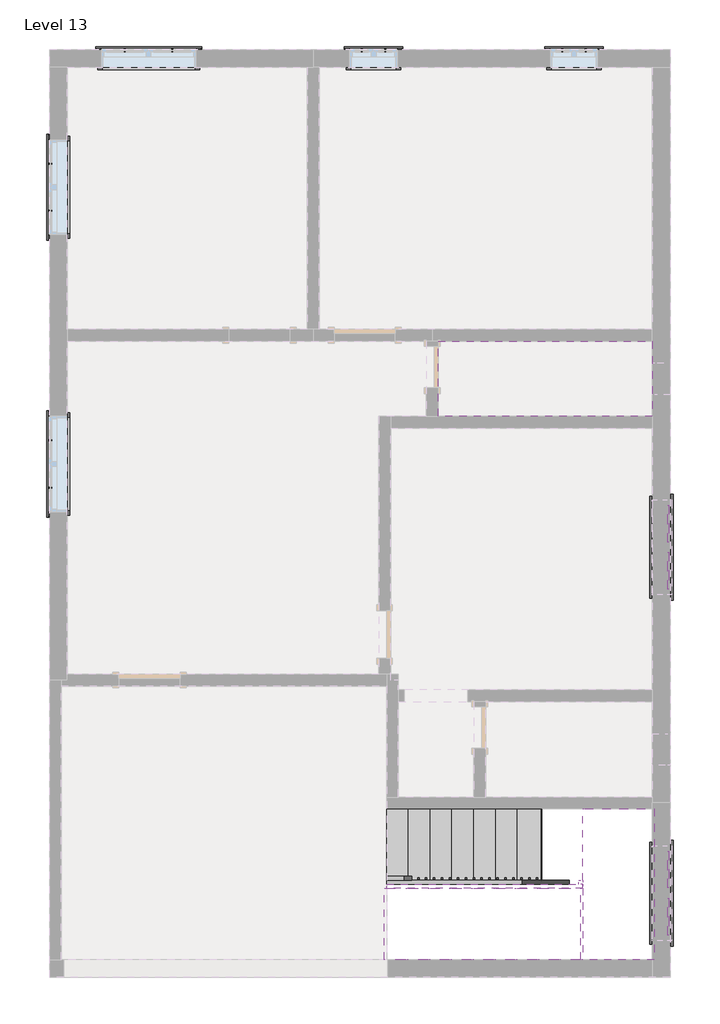
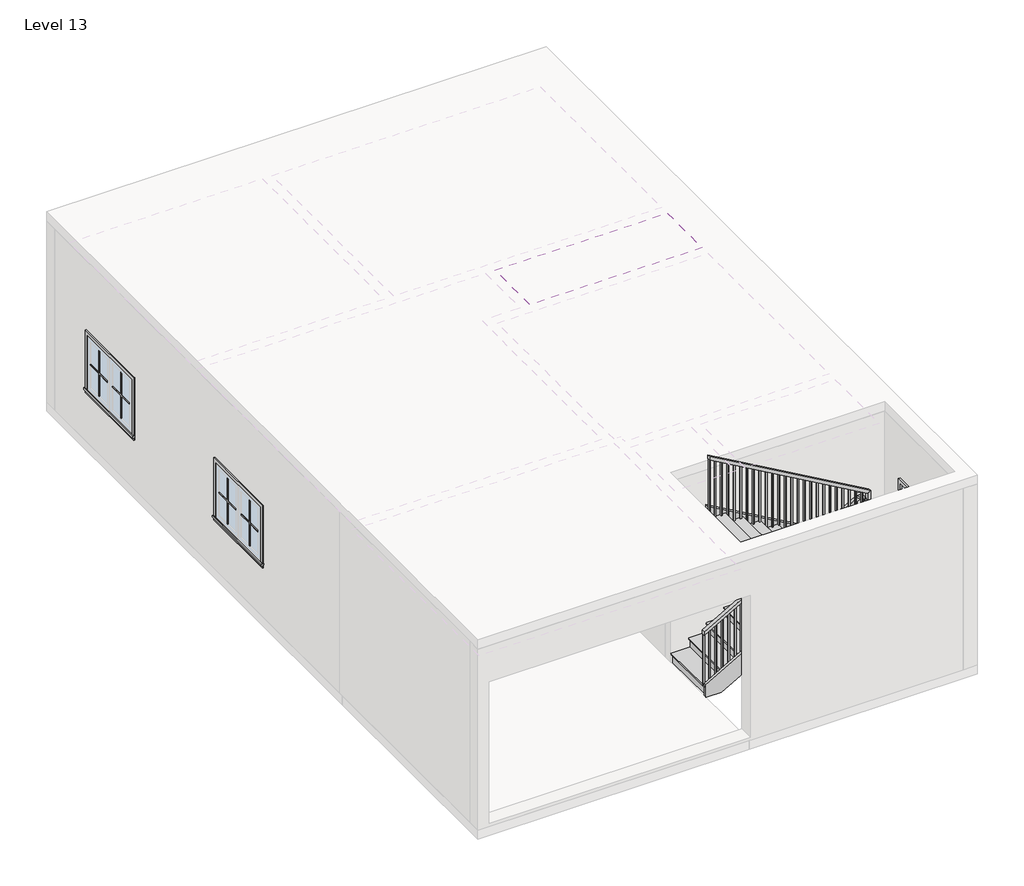
# One storey, part 2 of 2: 44 proxies, 3 members, 2 stair flights, 1 covering, 1 railing, 1 slab.
"""IFC4 building model written with IfcOpenShell, lengths in millimetres."""

from ifc_helpers import new_model, si_unit, frame, origin, place, context, project, spatial, polyline, outline, extrude, faceted_brep, transform, mapped, element, save
from components import muntin_pattern_2x2_muntin_pattern_2x2_2357e71d, muntin_pattern_2x2_muntin_pattern_2x2_302d8f29, muntin_pattern_2x2_muntin_pattern_2x2_53152e2c, muntin_pattern_2x2_muntin_pattern_2x2_e8f3e573, trim_window_exterior_flat_with_sill_c4e67c73, trim_window_exterior_flat_with_sill_a665a915, trim_window_interior_flat_picture_frame_cf1733af, trim_window_interior_flat_picture_frame_d485c387, non_monolithic_landing_4fb2f634, stair_flight_54a58d27, stair_flight_043378c7

model = new_model("IFC4")

# Units and contexts
model_context = context("Model", 3, world=origin())
ifc_project = project(units=[si_unit("LENGTHUNIT", "METRE", prefix="MILLI")], contexts=[model_context])

# Site, building, storey
site = spatial("IfcSite", under=ifc_project)
building = spatial("IfcBuilding", under=site)
storey = spatial("IfcBuildingStorey", under=building, Name="Level 13", Elevation=3200.4)

# Proxies
placement = place(None, origin())
muntin_pattern_2x2_muntin_pattern_2x2_shape = muntin_pattern_2x2_muntin_pattern_2x2_2357e71d(model_context)
element("IfcBuildingElementProxy", 1, Name="Muntin Pattern_2x2 : Muntin Pattern_2x2", ObjectType="Muntin Pattern_2x2 : Muntin Pattern_2x2", at=placement, inside=storey, context=model_context, shape_type="MappedRepresentation", body=[
    mapped(muntin_pattern_2x2_muntin_pattern_2x2_shape, transform((-4942.3279463, 5897.3080275, 4184.65), x_axis=(1.0, 0.0, 0.0), y_axis=(0.0, 1.0, 0.0), z_axis=(0.0, 0.0, 1.0))),
])
element("IfcBuildingElementProxy", 2, Name="Muntin Pattern_2x2 : Muntin Pattern_2x2", ObjectType="Muntin Pattern_2x2 : Muntin Pattern_2x2", at=placement, inside=storey, context=model_context, shape_type="MappedRepresentation", body=[
    mapped(muntin_pattern_2x2_muntin_pattern_2x2_shape, transform((-5899.5904463, 3838.3205275, 4184.65), x_axis=(0.0, 1.0, 0.0), y_axis=(-1.0, 0.0, 0.0), z_axis=(0.0, 0.0, 1.0))),
])
element("IfcBuildingElementProxy", 3, Name="Muntin Pattern_2x2 : Muntin Pattern_2x2", ObjectType="Muntin Pattern_2x2 : Muntin Pattern_2x2", at=placement, inside=storey, context=model_context, shape_type="MappedRepresentation", body=[
    mapped(muntin_pattern_2x2_muntin_pattern_2x2_shape, transform((-5899.5904463, 293.4330275, 4184.65), x_axis=(0.0, 1.0, 0.0), y_axis=(-1.0, 0.0, 0.0), z_axis=(0.0, 0.0, 1.0))),
])
element("IfcBuildingElementProxy", 4, Name="Muntin Pattern_2x2 : Muntin Pattern_2x2", ObjectType="Muntin Pattern_2x2 : Muntin Pattern_2x2", at=placement, inside=storey, context=model_context, shape_type="MappedRepresentation", body=[
    mapped(muntin_pattern_2x2_muntin_pattern_2x2_shape, transform((2031.5595537, -166.9419725, 4489.45), x_axis=(0.0, -1.0, 0.0), y_axis=(1.0, 0.0, 0.0), z_axis=(0.0, 0.0, 1.0))),
])
element("IfcBuildingElementProxy", 5, Name="Muntin Pattern_2x2 : Muntin Pattern_2x2", ObjectType="Muntin Pattern_2x2 : Muntin Pattern_2x2", at=placement, inside=storey, context=model_context, shape_type="MappedRepresentation", body=[
    mapped(muntin_pattern_2x2_muntin_pattern_2x2_shape, transform((2031.5595537, -4599.2419725, 4489.45), x_axis=(0.0, -1.0, 0.0), y_axis=(1.0, 0.0, 0.0), z_axis=(0.0, 0.0, 1.0))),
])
element("IfcBuildingElementProxy", 6, Name="Muntin Pattern_2x2 : Muntin Pattern_2x2", ObjectType="Muntin Pattern_2x2 : Muntin Pattern_2x2", at=placement, inside=storey, context=model_context, shape_type="MappedRepresentation", body=[
    mapped(muntin_pattern_2x2_muntin_pattern_2x2_shape, transform((-4942.3279463, 5897.3080275, 4184.65), x_axis=(1.0, 0.0, 0.0), y_axis=(0.0, 1.0, 0.0), z_axis=(0.0, 0.0, 1.0))),
])
element("IfcBuildingElementProxy", 7, Name="Muntin Pattern_2x2 : Muntin Pattern_2x2", ObjectType="Muntin Pattern_2x2 : Muntin Pattern_2x2", at=placement, inside=storey, context=model_context, shape_type="MappedRepresentation", body=[
    mapped(muntin_pattern_2x2_muntin_pattern_2x2_shape, transform((2031.5595537, -4599.2419725, 4489.45), x_axis=(0.0, -1.0, 0.0), y_axis=(1.0, 0.0, 0.0), z_axis=(0.0, 0.0, 1.0))),
])
muntin_pattern_2x2_muntin_pattern_2x2_2_shape = muntin_pattern_2x2_muntin_pattern_2x2_302d8f29(model_context)
element("IfcBuildingElementProxy", 8, Name="Muntin Pattern_2x2 : Muntin Pattern_2x2", ObjectType="Muntin Pattern_2x2 : Muntin Pattern_2x2", at=placement, inside=storey, context=model_context, shape_type="MappedRepresentation", body=[
    mapped(muntin_pattern_2x2_muntin_pattern_2x2_2_shape, transform((-4335.9029463, 5897.3080275, 4184.65), x_axis=(-1.0, 0.0, 0.0), y_axis=(0.0, -1.0, 0.0), z_axis=(0.0, 0.0, 1.0))),
])
element("IfcBuildingElementProxy", 9, Name="Muntin Pattern_2x2 : Muntin Pattern_2x2", ObjectType="Muntin Pattern_2x2 : Muntin Pattern_2x2", at=placement, inside=storey, context=model_context, shape_type="MappedRepresentation", body=[
    mapped(muntin_pattern_2x2_muntin_pattern_2x2_2_shape, transform((-5899.5904463, 4444.7455275, 4184.65), x_axis=(0.0, -1.0, 0.0), y_axis=(1.0, 0.0, 0.0), z_axis=(0.0, 0.0, 1.0))),
])
element("IfcBuildingElementProxy", 10, Name="Muntin Pattern_2x2 : Muntin Pattern_2x2", ObjectType="Muntin Pattern_2x2 : Muntin Pattern_2x2", at=placement, inside=storey, context=model_context, shape_type="MappedRepresentation", body=[
    mapped(muntin_pattern_2x2_muntin_pattern_2x2_2_shape, transform((-5899.5904463, 899.8580275, 4184.65), x_axis=(0.0, -1.0, 0.0), y_axis=(1.0, 0.0, 0.0), z_axis=(0.0, 0.0, 1.0))),
])
element("IfcBuildingElementProxy", 11, Name="Muntin Pattern_2x2 : Muntin Pattern_2x2", ObjectType="Muntin Pattern_2x2 : Muntin Pattern_2x2", at=placement, inside=storey, context=model_context, shape_type="MappedRepresentation", body=[
    mapped(muntin_pattern_2x2_muntin_pattern_2x2_2_shape, transform((2031.5595537, -773.3669725, 4489.45), x_axis=(0.0, 1.0, 0.0), y_axis=(-1.0, 0.0, 0.0), z_axis=(0.0, 0.0, 1.0))),
])
element("IfcBuildingElementProxy", 12, Name="Muntin Pattern_2x2 : Muntin Pattern_2x2", ObjectType="Muntin Pattern_2x2 : Muntin Pattern_2x2", at=placement, inside=storey, context=model_context, shape_type="MappedRepresentation", body=[
    mapped(muntin_pattern_2x2_muntin_pattern_2x2_2_shape, transform((2031.5595537, -5205.6669725, 4489.45), x_axis=(0.0, 1.0, 0.0), y_axis=(-1.0, 0.0, 0.0), z_axis=(0.0, 0.0, 1.0))),
])
element("IfcBuildingElementProxy", 13, Name="Muntin Pattern_2x2 : Muntin Pattern_2x2", ObjectType="Muntin Pattern_2x2 : Muntin Pattern_2x2", at=placement, inside=storey, context=model_context, shape_type="MappedRepresentation", body=[
    mapped(muntin_pattern_2x2_muntin_pattern_2x2_2_shape, transform((-4335.9029463, 5897.3080275, 4184.65), x_axis=(-1.0, 0.0, 0.0), y_axis=(0.0, -1.0, 0.0), z_axis=(0.0, 0.0, 1.0))),
])
element("IfcBuildingElementProxy", 14, Name="Muntin Pattern_2x2 : Muntin Pattern_2x2", ObjectType="Muntin Pattern_2x2 : Muntin Pattern_2x2", at=placement, inside=storey, context=model_context, shape_type="MappedRepresentation", body=[
    mapped(muntin_pattern_2x2_muntin_pattern_2x2_2_shape, transform((2031.5595537, -5205.6669725, 4489.45), x_axis=(0.0, 1.0, 0.0), y_axis=(-1.0, 0.0, 0.0), z_axis=(0.0, 0.0, 1.0))),
])
muntin_pattern_2x2_muntin_pattern_2x2_3_shape = muntin_pattern_2x2_muntin_pattern_2x2_53152e2c(model_context)
element("IfcBuildingElementProxy", 15, Name="Muntin Pattern_2x2 : Muntin Pattern_2x2", ObjectType="Muntin Pattern_2x2 : Muntin Pattern_2x2", at=placement, inside=storey, context=model_context, shape_type="MappedRepresentation", body=[
    mapped(muntin_pattern_2x2_muntin_pattern_2x2_3_shape, transform((-1907.0279463, 5897.3080275, 4184.65), x_axis=(1.0, 0.0, 0.0), y_axis=(0.0, 1.0, 0.0), z_axis=(0.0, 0.0, 1.0))),
])
element("IfcBuildingElementProxy", 16, Name="Muntin Pattern_2x2 : Muntin Pattern_2x2", ObjectType="Muntin Pattern_2x2 : Muntin Pattern_2x2", at=placement, inside=storey, context=model_context, shape_type="MappedRepresentation", body=[
    mapped(muntin_pattern_2x2_muntin_pattern_2x2_3_shape, transform((658.3720537, 5897.3080275, 4184.65), x_axis=(1.0, 0.0, 0.0), y_axis=(0.0, 1.0, 0.0), z_axis=(0.0, 0.0, 1.0))),
])
element("IfcBuildingElementProxy", 17, Name="Muntin Pattern_2x2 : Muntin Pattern_2x2", ObjectType="Muntin Pattern_2x2 : Muntin Pattern_2x2", at=placement, inside=storey, context=model_context, shape_type="MappedRepresentation", body=[
    mapped(muntin_pattern_2x2_muntin_pattern_2x2_3_shape, transform((-1907.0279463, 5897.3080275, 4184.65), x_axis=(1.0, 0.0, 0.0), y_axis=(0.0, 1.0, 0.0), z_axis=(0.0, 0.0, 1.0))),
])
element("IfcBuildingElementProxy", 18, Name="Muntin Pattern_2x2 : Muntin Pattern_2x2", ObjectType="Muntin Pattern_2x2 : Muntin Pattern_2x2", at=placement, inside=storey, context=model_context, shape_type="MappedRepresentation", body=[
    mapped(muntin_pattern_2x2_muntin_pattern_2x2_3_shape, transform((658.3720537, 5897.3080275, 4184.65), x_axis=(1.0, 0.0, 0.0), y_axis=(0.0, 1.0, 0.0), z_axis=(0.0, 0.0, 1.0))),
])
muntin_pattern_2x2_muntin_pattern_2x2_4_shape = muntin_pattern_2x2_muntin_pattern_2x2_e8f3e573(model_context)
element("IfcBuildingElementProxy", 19, Name="Muntin Pattern_2x2 : Muntin Pattern_2x2", ObjectType="Muntin Pattern_2x2 : Muntin Pattern_2x2", at=placement, inside=storey, context=model_context, shape_type="MappedRepresentation", body=[
    mapped(muntin_pattern_2x2_muntin_pattern_2x2_4_shape, transform((-1605.4029463, 5897.3080275, 4184.65), x_axis=(-1.0, 0.0, 0.0), y_axis=(0.0, -1.0, 0.0), z_axis=(0.0, 0.0, 1.0))),
])
element("IfcBuildingElementProxy", 20, Name="Muntin Pattern_2x2 : Muntin Pattern_2x2", ObjectType="Muntin Pattern_2x2 : Muntin Pattern_2x2", at=placement, inside=storey, context=model_context, shape_type="MappedRepresentation", body=[
    mapped(muntin_pattern_2x2_muntin_pattern_2x2_4_shape, transform((959.9970537, 5897.3080275, 4184.65), x_axis=(-1.0, 0.0, 0.0), y_axis=(0.0, -1.0, 0.0), z_axis=(0.0, 0.0, 1.0))),
])
element("IfcBuildingElementProxy", 21, Name="Muntin Pattern_2x2 : Muntin Pattern_2x2", ObjectType="Muntin Pattern_2x2 : Muntin Pattern_2x2", at=placement, inside=storey, context=model_context, shape_type="MappedRepresentation", body=[
    mapped(muntin_pattern_2x2_muntin_pattern_2x2_4_shape, transform((-1605.4029463, 5897.3080275, 4184.65), x_axis=(-1.0, 0.0, 0.0), y_axis=(0.0, -1.0, 0.0), z_axis=(0.0, 0.0, 1.0))),
])
element("IfcBuildingElementProxy", 22, Name="Muntin Pattern_2x2 : Muntin Pattern_2x2", ObjectType="Muntin Pattern_2x2 : Muntin Pattern_2x2", at=placement, inside=storey, context=model_context, shape_type="MappedRepresentation", body=[
    mapped(muntin_pattern_2x2_muntin_pattern_2x2_4_shape, transform((959.9970537, 5897.3080275, 4184.65), x_axis=(-1.0, 0.0, 0.0), y_axis=(0.0, -1.0, 0.0), z_axis=(0.0, 0.0, 1.0))),
])
trim_window_exterior_flat_with_sill_shape = trim_window_exterior_flat_with_sill_c4e67c73(model_context)
element("IfcBuildingElementProxy", 23, Name="Trim-Window-Exterior-Flat : with Sill", ObjectType="Trim-Window-Exterior-Flat : with Sill", at=placement, inside=storey, context=model_context, shape_type="MappedRepresentation", body=[
    mapped(trim_window_exterior_flat_with_sill_shape, transform((-4639.1154463, 5906.8330275, 5029.2), x_axis=(-1.0, 0.0, 0.0), y_axis=(0.0, 0.0, 1.0), z_axis=(0.0, 1.0, 0.0))),
])
element("IfcBuildingElementProxy", 24, Name="Trim-Window-Exterior-Flat : with Sill", ObjectType="Trim-Window-Exterior-Flat : with Sill", at=placement, inside=storey, context=model_context, shape_type="MappedRepresentation", body=[
    mapped(trim_window_exterior_flat_with_sill_shape, transform((-5909.1154463, 4141.5330275, 5029.2), x_axis=(0.0, -1.0, 0.0), y_axis=(0.0, 0.0, 1.0), z_axis=(-1.0, 0.0, 0.0))),
])
element("IfcBuildingElementProxy", 25, Name="Trim-Window-Exterior-Flat : with Sill", ObjectType="Trim-Window-Exterior-Flat : with Sill", at=placement, inside=storey, context=model_context, shape_type="MappedRepresentation", body=[
    mapped(trim_window_exterior_flat_with_sill_shape, transform((-5909.1154463, 596.6455275, 5029.2), x_axis=(0.0, -1.0, 0.0), y_axis=(0.0, 0.0, 1.0), z_axis=(-1.0, 0.0, 0.0))),
])
element("IfcBuildingElementProxy", 26, Name="Trim-Window-Exterior-Flat : with Sill", ObjectType="Trim-Window-Exterior-Flat : with Sill", at=placement, inside=storey, context=model_context, shape_type="MappedRepresentation", body=[
    mapped(trim_window_exterior_flat_with_sill_shape, transform((2041.0845537, -470.1544725, 5334.0), x_axis=(0.0, 1.0, 0.0), y_axis=(0.0, 0.0, 1.0), z_axis=(1.0, 0.0, 0.0))),
])
element("IfcBuildingElementProxy", 27, Name="Trim-Window-Exterior-Flat : with Sill", ObjectType="Trim-Window-Exterior-Flat : with Sill", at=placement, inside=storey, context=model_context, shape_type="MappedRepresentation", body=[
    mapped(trim_window_exterior_flat_with_sill_shape, transform((2041.0845537, -4902.4544725, 5334.0), x_axis=(0.0, 1.0, 0.0), y_axis=(0.0, 0.0, 1.0), z_axis=(1.0, 0.0, 0.0))),
])
element("IfcBuildingElementProxy", 28, Name="Trim-Window-Exterior-Flat : with Sill", ObjectType="Trim-Window-Exterior-Flat : with Sill", at=placement, inside=storey, context=model_context, shape_type="MappedRepresentation", body=[
    mapped(trim_window_exterior_flat_with_sill_shape, transform((-4639.1154463, 5906.8330275, 5029.2), x_axis=(-1.0, 0.0, 0.0), y_axis=(0.0, 0.0, 1.0), z_axis=(0.0, 1.0, 0.0))),
])
element("IfcBuildingElementProxy", 29, Name="Trim-Window-Exterior-Flat : with Sill", ObjectType="Trim-Window-Exterior-Flat : with Sill", at=placement, inside=storey, context=model_context, shape_type="MappedRepresentation", body=[
    mapped(trim_window_exterior_flat_with_sill_shape, transform((2041.0845537, -4902.4544725, 5334.0), x_axis=(0.0, 1.0, 0.0), y_axis=(0.0, 0.0, 1.0), z_axis=(1.0, 0.0, 0.0))),
])
trim_window_exterior_flat_with_sill_2_shape = trim_window_exterior_flat_with_sill_a665a915(model_context)
element("IfcBuildingElementProxy", 30, Name="Trim-Window-Exterior-Flat : with Sill", ObjectType="Trim-Window-Exterior-Flat : with Sill", at=placement, inside=storey, context=model_context, shape_type="MappedRepresentation", body=[
    mapped(trim_window_exterior_flat_with_sill_2_shape, transform((-1756.2154463, 5906.8330275, 5029.2), x_axis=(-1.0, 0.0, 0.0), y_axis=(0.0, 0.0, 1.0), z_axis=(0.0, 1.0, 0.0))),
])
element("IfcBuildingElementProxy", 31, Name="Trim-Window-Exterior-Flat : with Sill", ObjectType="Trim-Window-Exterior-Flat : with Sill", at=placement, inside=storey, context=model_context, shape_type="MappedRepresentation", body=[
    mapped(trim_window_exterior_flat_with_sill_2_shape, transform((809.1845537, 5906.8330275, 5029.2), x_axis=(-1.0, 0.0, 0.0), y_axis=(0.0, 0.0, 1.0), z_axis=(0.0, 1.0, 0.0))),
])
element("IfcBuildingElementProxy", 32, Name="Trim-Window-Exterior-Flat : with Sill", ObjectType="Trim-Window-Exterior-Flat : with Sill", at=placement, inside=storey, context=model_context, shape_type="MappedRepresentation", body=[
    mapped(trim_window_exterior_flat_with_sill_2_shape, transform((-1756.2154463, 5906.8330275, 5029.2), x_axis=(-1.0, 0.0, 0.0), y_axis=(0.0, 0.0, 1.0), z_axis=(0.0, 1.0, 0.0))),
])
element("IfcBuildingElementProxy", 33, Name="Trim-Window-Exterior-Flat : with Sill", ObjectType="Trim-Window-Exterior-Flat : with Sill", at=placement, inside=storey, context=model_context, shape_type="MappedRepresentation", body=[
    mapped(trim_window_exterior_flat_with_sill_2_shape, transform((809.1845537, 5906.8330275, 5029.2), x_axis=(-1.0, 0.0, 0.0), y_axis=(0.0, 0.0, 1.0), z_axis=(0.0, 1.0, 0.0))),
])
trim_window_interior_flat_picture_frame_shape = trim_window_interior_flat_picture_frame_cf1733af(model_context)
element("IfcBuildingElementProxy", 34, Name="Trim-Window-Interior-Flat : Picture Frame", ObjectType="Trim-Window-Interior-Flat : Picture Frame", at=placement, inside=storey, context=model_context, shape_type="MappedRepresentation", body=[
    mapped(trim_window_interior_flat_picture_frame_shape, transform((-4639.1154463, 5678.2330275, 5029.2), x_axis=(1.0, 0.0, 0.0), y_axis=(0.0, 0.0, 1.0), z_axis=(0.0, -1.0, 0.0))),
])
element("IfcBuildingElementProxy", 35, Name="Trim-Window-Interior-Flat : Picture Frame", ObjectType="Trim-Window-Interior-Flat : Picture Frame", at=placement, inside=storey, context=model_context, shape_type="MappedRepresentation", body=[
    mapped(trim_window_interior_flat_picture_frame_shape, transform((-5680.5154463, 4141.5330275, 5029.2), x_axis=(0.0, 1.0, 0.0), y_axis=(0.0, 0.0, 1.0), z_axis=(1.0, 0.0, 0.0))),
])
element("IfcBuildingElementProxy", 36, Name="Trim-Window-Interior-Flat : Picture Frame", ObjectType="Trim-Window-Interior-Flat : Picture Frame", at=placement, inside=storey, context=model_context, shape_type="MappedRepresentation", body=[
    mapped(trim_window_interior_flat_picture_frame_shape, transform((-5680.5154463, 596.6455275, 5029.2), x_axis=(0.0, 1.0, 0.0), y_axis=(0.0, 0.0, 1.0), z_axis=(1.0, 0.0, 0.0))),
])
element("IfcBuildingElementProxy", 37, Name="Trim-Window-Interior-Flat : Picture Frame", ObjectType="Trim-Window-Interior-Flat : Picture Frame", at=placement, inside=storey, context=model_context, shape_type="MappedRepresentation", body=[
    mapped(trim_window_interior_flat_picture_frame_shape, transform((1812.4845537, -470.1544725, 5334.0), x_axis=(0.0, -1.0, 0.0), y_axis=(0.0, 0.0, 1.0), z_axis=(-1.0, 0.0, 0.0))),
])
element("IfcBuildingElementProxy", 38, Name="Trim-Window-Interior-Flat : Picture Frame", ObjectType="Trim-Window-Interior-Flat : Picture Frame", at=placement, inside=storey, context=model_context, shape_type="MappedRepresentation", body=[
    mapped(trim_window_interior_flat_picture_frame_shape, transform((1812.4845537, -4902.4544725, 5334.0), x_axis=(0.0, -1.0, 0.0), y_axis=(0.0, 0.0, 1.0), z_axis=(-1.0, 0.0, 0.0))),
])
element("IfcBuildingElementProxy", 39, Name="Trim-Window-Interior-Flat : Picture Frame", ObjectType="Trim-Window-Interior-Flat : Picture Frame", at=placement, inside=storey, context=model_context, shape_type="MappedRepresentation", body=[
    mapped(trim_window_interior_flat_picture_frame_shape, transform((-4639.1154463, 5678.2330275, 5029.2), x_axis=(1.0, 0.0, 0.0), y_axis=(0.0, 0.0, 1.0), z_axis=(0.0, -1.0, 0.0))),
])
element("IfcBuildingElementProxy", 40, Name="Trim-Window-Interior-Flat : Picture Frame", ObjectType="Trim-Window-Interior-Flat : Picture Frame", at=placement, inside=storey, context=model_context, shape_type="MappedRepresentation", body=[
    mapped(trim_window_interior_flat_picture_frame_shape, transform((1812.4845537, -4902.4544725, 5334.0), x_axis=(0.0, -1.0, 0.0), y_axis=(0.0, 0.0, 1.0), z_axis=(-1.0, 0.0, 0.0))),
])
trim_window_interior_flat_picture_frame_2_shape = trim_window_interior_flat_picture_frame_d485c387(model_context)
element("IfcBuildingElementProxy", 41, Name="Trim-Window-Interior-Flat : Picture Frame", ObjectType="Trim-Window-Interior-Flat : Picture Frame", at=placement, inside=storey, context=model_context, shape_type="MappedRepresentation", body=[
    mapped(trim_window_interior_flat_picture_frame_2_shape, transform((-1756.2154463, 5678.2330275, 5029.2), x_axis=(1.0, 0.0, 0.0), y_axis=(0.0, 0.0, 1.0), z_axis=(0.0, -1.0, 0.0))),
])
element("IfcBuildingElementProxy", 42, Name="Trim-Window-Interior-Flat : Picture Frame", ObjectType="Trim-Window-Interior-Flat : Picture Frame", at=placement, inside=storey, context=model_context, shape_type="MappedRepresentation", body=[
    mapped(trim_window_interior_flat_picture_frame_2_shape, transform((809.1845537, 5678.2330275, 5029.2), x_axis=(1.0, 0.0, 0.0), y_axis=(0.0, 0.0, 1.0), z_axis=(0.0, -1.0, 0.0))),
])
element("IfcBuildingElementProxy", 43, Name="Trim-Window-Interior-Flat : Picture Frame", ObjectType="Trim-Window-Interior-Flat : Picture Frame", at=placement, inside=storey, context=model_context, shape_type="MappedRepresentation", body=[
    mapped(trim_window_interior_flat_picture_frame_2_shape, transform((-1756.2154463, 5678.2330275, 5029.2), x_axis=(1.0, 0.0, 0.0), y_axis=(0.0, 0.0, 1.0), z_axis=(0.0, -1.0, 0.0))),
])
element("IfcBuildingElementProxy", 44, Name="Trim-Window-Interior-Flat : Picture Frame", ObjectType="Trim-Window-Interior-Flat : Picture Frame", at=placement, inside=storey, context=model_context, shape_type="MappedRepresentation", body=[
    mapped(trim_window_interior_flat_picture_frame_2_shape, transform((809.1845537, 5678.2330275, 5029.2), x_axis=(1.0, 0.0, 0.0), y_axis=(0.0, 0.0, 1.0), z_axis=(0.0, -1.0, 0.0))),
])

# Covering
element("IfcCovering", 45, ObjectType="2' x 4' ACT System", at=placement, inside=storey, context=model_context, shape_type="SweptSolid", body=[
    extrude(outline(polyline([(-930.7154463, 2171.4455275), (1812.4845537, 2171.4455275), (1812.4845537, 1206.2455275), (-930.7154463, 1206.2455275), (-930.7154463, 2171.4455275)])), frame((0.0, 0.0, 5943.6), z_axis=(0.0, 0.0, 1.0), x_axis=(1.0, 0.0, 0.0)), (0.0, 0.0, 1.0), 57.15),
])

# Members
element("IfcMember", 46, ObjectType="Stringer - 2\" Width", at=placement, inside=storey, context=model_context, shape_type="SweptSolid", body=[
    extrude(outline(polyline([(3409.4890626, -1591.1154463), (3200.4, -1591.1154463), (3200.4, -1342.8974141), (4469.324218, 872.6845537), (4820.5745172, 872.6845537), (3409.4890626, -1591.1154463)])), frame((0.0, -4788.1544725, 0.0), z_axis=(0.0, 1.0, 0.0), x_axis=(0.0, 0.0, 1.0)), (0.0, 0.0, 1.0), 50.8),
])
element("IfcMember", 47, ObjectType="Stringer - 2\" Width", at=placement, inside=storey, context=model_context, shape_type="SweptSolid", body=[
    extrude(outline(polyline([(4658.4387634, 923.4845537), (5009.6890626, 923.4845537), (6449.8690626, -1591.1154463), (6098.6187634, -1591.1154463), (4658.4387634, 923.4845537)])), frame((0.0, -4838.9544725, 0.0), z_axis=(0.0, 1.0, 0.0), x_axis=(0.0, 0.0, 1.0)), (0.0, 0.0, 1.0), 50.8),
])
element("IfcMember", 48, ObjectType="Stringer - 2\" Width", at=placement, inside=storey, context=model_context, shape_type="SweptSolid", body=[
    extrude(outline(polyline([(872.6845537, -4737.3544725), (923.4845537, -4737.3544725), (923.4845537, -4788.1544725), (872.6845537, -4788.1544725), (872.6845537, -4737.3544725)])), frame((0.0, 0.0, 4572.0), z_axis=(0.0, 0.0, 1.0), x_axis=(1.0, 0.0, 0.0)), (0.0, 0.0, 1.0), 304.8),
])

# Railing
element("IfcRailing", 49, ObjectType="Handrail - Rectangular", at=placement, inside=storey, context=model_context, shape_type="SolidModel", body=[
    faceted_brep([(-1591.1154463, -4686.5544725, 4274.82), (-1591.1154463, -4686.5544725, 4216.2782835), (-1591.1154463, -4737.3544725, 4216.2782835), (-1591.1154463, -4737.3544725, 4274.82), (847.2845537, -4686.5544725, 5671.3581818), (898.0845537, -4686.5544725, 5641.9110107), (898.0845537, -4737.3544725, 5641.9110107), (847.2845537, -4737.3544725, 5671.3581818), (847.2845537, -4686.5544725, 5715.0), (898.0845537, -4686.5544725, 5664.2), (898.0845537, -4737.3544725, 5664.2), (847.2845537, -4737.3544725, 5715.0), (974.2845537, -4686.5544725, 5715.0), (974.2845537, -4686.5544725, 5664.2), (923.4845537, -4737.3544725, 5664.2), (923.4845537, -4737.3544725, 5715.0), (974.2845537, -4813.5544725, 5715.0), (974.2845537, -4813.5544725, 5664.2), (923.4845537, -4813.5544725, 5664.2), (923.4845537, -4813.5544725, 5715.0), (974.2845537, -4838.9544725, 5715.0), (923.4845537, -4838.9544725, 5715.0), (923.4845537, -4889.7544725, 5664.2), (974.2845537, -4889.7544725, 5664.2)], [[[0, 1, 2, 3]], [[1, 0, 4, 5]], [[2, 1, 5, 6]], [[3, 2, 6, 7]], [[0, 3, 7, 4]], [[5, 4, 8, 9]], [[6, 5, 9, 10]], [[7, 6, 10, 11]], [[4, 7, 11, 8]], [[9, 8, 12, 13]], [[10, 9, 13, 14]], [[11, 10, 14, 15]], [[8, 11, 15, 12]], [[13, 12, 16, 17]], [[14, 13, 17, 18]], [[15, 14, 18, 19]], [[12, 15, 19, 16]], [[20, 21, 22, 23]], [[17, 16, 20, 23]], [[18, 17, 23, 22]], [[19, 18, 22, 21]], [[16, 19, 21, 20]]]),
    faceted_brep([(974.2845537, -4838.9544725, 5715.0), (974.2845537, -4889.7544725, 5664.2), (923.4845537, -4889.7544725, 5664.2), (923.4845537, -4838.9544725, 5715.0), (974.2845537, -4838.9544725, 5845.9254545), (923.4845537, -4838.9544725, 5816.4782835), (923.4845537, -4889.7544725, 5816.4782835), (974.2845537, -4889.7544725, 5845.9254545)], [[[0, 1, 2, 3]], [[4, 5, 6, 7]], [[1, 0, 4, 7]], [[2, 1, 7, 6]], [[3, 2, 6, 5]], [[0, 3, 5, 4]]]),
    faceted_brep([(974.2845537, -4889.7544725, 5845.9254545), (923.4845537, -4889.7544725, 5816.4782835), (923.4845537, -4838.9544725, 5816.4782835), (974.2845537, -4838.9544725, 5845.9254545), (-1591.1154463, -4889.7544725, 7315.2), (-1591.1154463, -4838.9544725, 7315.2), (-1591.1154463, -4838.9544725, 7256.6582835), (-1591.1154463, -4889.7544725, 7256.6582835)], [[[0, 1, 2, 3]], [[4, 5, 6, 7]], [[1, 0, 4, 7]], [[2, 1, 7, 6]], [[3, 2, 6, 5]], [[0, 3, 5, 4]]]),
    extrude(outline(polyline([(7193.0139653, -1479.9904463), (7203.9244198, -1499.0404463), (6240.78, -1499.0404463), (6240.78, -1479.9904463), (7193.0139653, -1479.9904463)])), frame((0.0, -4873.8794725, 0.0), z_axis=(0.0, 1.0, 0.0), x_axis=(0.0, 0.0, 1.0)), (0.0, 0.0, 1.0), 19.05),
    extrude(outline(polyline([(7134.8248744, -1378.3904463), (7145.7353289, -1397.4404463), (6240.78, -1397.4404463), (6240.78, -1378.3904463), (7134.8248744, -1378.3904463)])), frame((0.0, -4873.8794725, 0.0), z_axis=(0.0, 1.0, 0.0), x_axis=(0.0, 0.0, 1.0)), (0.0, 0.0, 1.0), 19.05),
    extrude(outline(polyline([(7076.6357835, -1276.7904463), (7087.546238, -1295.8404463), (6080.76, -1295.8404463), (6080.76, -1276.7904463), (7076.6357835, -1276.7904463)])), frame((0.0, -4873.8794725, 0.0), z_axis=(0.0, 1.0, 0.0), x_axis=(0.0, 0.0, 1.0)), (0.0, 0.0, 1.0), 19.05),
    extrude(outline(polyline([(7018.4466926, -1175.1904463), (7029.3571471, -1194.2404463), (6080.76, -1194.2404463), (6080.76, -1175.1904463), (7018.4466926, -1175.1904463)])), frame((0.0, -4873.8794725, 0.0), z_axis=(0.0, 1.0, 0.0), x_axis=(0.0, 0.0, 1.0)), (0.0, 0.0, 1.0), 19.05),
    extrude(outline(polyline([(6960.2576016, -1073.5904463), (6971.1680562, -1092.6404463), (6080.76, -1092.6404463), (6080.76, -1073.5904463), (6960.2576016, -1073.5904463)])), frame((0.0, -4873.8794725, 0.0), z_axis=(0.0, 1.0, 0.0), x_axis=(0.0, 0.0, 1.0)), (0.0, 0.0, 1.0), 19.05),
    extrude(outline(polyline([(6902.0685107, -971.9904463), (6912.9789653, -991.0404463), (5920.74, -991.0404463), (5920.74, -971.9904463), (6902.0685107, -971.9904463)])), frame((0.0, -4873.8794725, 0.0), z_axis=(0.0, 1.0, 0.0), x_axis=(0.0, 0.0, 1.0)), (0.0, 0.0, 1.0), 19.05),
    extrude(outline(polyline([(6843.8794198, -870.3904463), (6854.7898744, -889.4404463), (5920.74, -889.4404463), (5920.74, -870.3904463), (6843.8794198, -870.3904463)])), frame((0.0, -4873.8794725, 0.0), z_axis=(0.0, 1.0, 0.0), x_axis=(0.0, 0.0, 1.0)), (0.0, 0.0, 1.0), 19.05),
    extrude(outline(polyline([(6785.6903289, -768.7904463), (6796.6007835, -787.8404463), (5920.74, -787.8404463), (5920.74, -768.7904463), (6785.6903289, -768.7904463)])), frame((0.0, -4873.8794725, 0.0), z_axis=(0.0, 1.0, 0.0), x_axis=(0.0, 0.0, 1.0)), (0.0, 0.0, 1.0), 19.05),
    extrude(outline(polyline([(6727.501238, -667.1904463), (6738.4116926, -686.2404463), (5760.72, -686.2404463), (5760.72, -667.1904463), (6727.501238, -667.1904463)])), frame((0.0, -4873.8794725, 0.0), z_axis=(0.0, 1.0, 0.0), x_axis=(0.0, 0.0, 1.0)), (0.0, 0.0, 1.0), 19.05),
    extrude(outline(polyline([(6669.3121471, -565.5904463), (6680.2226016, -584.6404463), (5760.72, -584.6404463), (5760.72, -565.5904463), (6669.3121471, -565.5904463)])), frame((0.0, -4873.8794725, 0.0), z_axis=(0.0, 1.0, 0.0), x_axis=(0.0, 0.0, 1.0)), (0.0, 0.0, 1.0), 19.05),
    extrude(outline(polyline([(6611.1230562, -463.9904463), (6622.0335107, -483.0404463), (5760.72, -483.0404463), (5760.72, -463.9904463), (6611.1230562, -463.9904463)])), frame((0.0, -4873.8794725, 0.0), z_axis=(0.0, 1.0, 0.0), x_axis=(0.0, 0.0, 1.0)), (0.0, 0.0, 1.0), 19.05),
    extrude(outline(polyline([(6552.9339653, -362.3904463), (6563.8444198, -381.4404463), (5600.7, -381.4404463), (5600.7, -362.3904463), (6552.9339653, -362.3904463)])), frame((0.0, -4873.8794725, 0.0), z_axis=(0.0, 1.0, 0.0), x_axis=(0.0, 0.0, 1.0)), (0.0, 0.0, 1.0), 19.05),
    extrude(outline(polyline([(6494.7448744, -260.7904463), (6505.6553289, -279.8404463), (5600.7, -279.8404463), (5600.7, -260.7904463), (6494.7448744, -260.7904463)])), frame((0.0, -4873.8794725, 0.0), z_axis=(0.0, 1.0, 0.0), x_axis=(0.0, 0.0, 1.0)), (0.0, 0.0, 1.0), 19.05),
    extrude(outline(polyline([(6436.5557835, -159.1904463), (6447.466238, -178.2404463), (5440.68, -178.2404463), (5440.68, -159.1904463), (6436.5557835, -159.1904463)])), frame((0.0, -4873.8794725, 0.0), z_axis=(0.0, 1.0, 0.0), x_axis=(0.0, 0.0, 1.0)), (0.0, 0.0, 1.0), 19.05),
    extrude(outline(polyline([(6378.3666926, -57.5904463), (6389.2771471, -76.6404463), (5440.68, -76.6404463), (5440.68, -57.5904463), (6378.3666926, -57.5904463)])), frame((0.0, -4873.8794725, 0.0), z_axis=(0.0, 1.0, 0.0), x_axis=(0.0, 0.0, 1.0)), (0.0, 0.0, 1.0), 19.05),
    extrude(outline(polyline([(6320.1776016, 44.0095537), (6331.0880562, 24.9595537), (5440.68, 24.9595537), (5440.68, 44.0095537), (6320.1776016, 44.0095537)])), frame((0.0, -4873.8794725, 0.0), z_axis=(0.0, 1.0, 0.0), x_axis=(0.0, 0.0, 1.0)), (0.0, 0.0, 1.0), 19.05),
    extrude(outline(polyline([(6261.9885107, 145.6095537), (6272.8989653, 126.5595537), (5280.66, 126.5595537), (5280.66, 145.6095537), (6261.9885107, 145.6095537)])), frame((0.0, -4873.8794725, 0.0), z_axis=(0.0, 1.0, 0.0), x_axis=(0.0, 0.0, 1.0)), (0.0, 0.0, 1.0), 19.05),
    extrude(outline(polyline([(6203.7994198, 247.2095537), (6214.7098744, 228.1595537), (5280.66, 228.1595537), (5280.66, 247.2095537), (6203.7994198, 247.2095537)])), frame((0.0, -4873.8794725, 0.0), z_axis=(0.0, 1.0, 0.0), x_axis=(0.0, 0.0, 1.0)), (0.0, 0.0, 1.0), 19.05),
    extrude(outline(polyline([(6145.6103289, 348.8095537), (6156.5207835, 329.7595537), (5280.66, 329.7595537), (5280.66, 348.8095537), (6145.6103289, 348.8095537)])), frame((0.0, -4873.8794725, 0.0), z_axis=(0.0, 1.0, 0.0), x_axis=(0.0, 0.0, 1.0)), (0.0, 0.0, 1.0), 19.05),
    extrude(outline(polyline([(6087.421238, 450.4095537), (6098.3316926, 431.3595537), (5120.64, 431.3595537), (5120.64, 450.4095537), (6087.421238, 450.4095537)])), frame((0.0, -4873.8794725, 0.0), z_axis=(0.0, 1.0, 0.0), x_axis=(0.0, 0.0, 1.0)), (0.0, 0.0, 1.0), 19.05),
    extrude(outline(polyline([(6029.2321471, 552.0095537), (6040.1426016, 532.9595537), (5120.64, 532.9595537), (5120.64, 552.0095537), (6029.2321471, 552.0095537)])), frame((0.0, -4873.8794725, 0.0), z_axis=(0.0, 1.0, 0.0), x_axis=(0.0, 0.0, 1.0)), (0.0, 0.0, 1.0), 19.05),
    extrude(outline(polyline([(5971.0430562, 653.6095537), (5981.9535107, 634.5595537), (5120.64, 634.5595537), (5120.64, 653.6095537), (5971.0430562, 653.6095537)])), frame((0.0, -4873.8794725, 0.0), z_axis=(0.0, 1.0, 0.0), x_axis=(0.0, 0.0, 1.0)), (0.0, 0.0, 1.0), 19.05),
    extrude(outline(polyline([(5912.8539653, 755.2095537), (5923.7644198, 736.1595537), (4960.62, 736.1595537), (4960.62, 755.2095537), (5912.8539653, 755.2095537)])), frame((0.0, -4873.8794725, 0.0), z_axis=(0.0, 1.0, 0.0), x_axis=(0.0, 0.0, 1.0)), (0.0, 0.0, 1.0), 19.05),
    extrude(outline(polyline([(5854.6648744, 856.8095537), (5865.5753289, 837.7595537), (4960.62, 837.7595537), (4960.62, 856.8095537), (5854.6648744, 856.8095537)])), frame((0.0, -4873.8794725, 0.0), z_axis=(0.0, 1.0, 0.0), x_axis=(0.0, 0.0, 1.0)), (0.0, 0.0, 1.0), 19.05),
    extrude(outline(polyline([(939.3595537, -4804.0294725), (958.4095537, -4804.0294725), (958.4095537, -4823.0794725), (939.3595537, -4823.0794725), (939.3595537, -4804.0294725)])), frame((0.0, 0.0, 4800.6), z_axis=(0.0, 0.0, 1.0), x_axis=(1.0, 0.0, 0.0)), (0.0, 0.0, 1.0), 863.6),
    extrude(outline(polyline([(5618.2716926, 856.8095537), (5607.361238, 837.7595537), (4640.58, 837.7595537), (4640.58, 856.8095537), (5618.2716926, 856.8095537)])), frame((0.0, -4721.4794725, 0.0), z_axis=(0.0, 1.0, 0.0), x_axis=(0.0, 0.0, 1.0)), (0.0, 0.0, 1.0), 19.05),
    extrude(outline(polyline([(5560.0826016, 755.2095537), (5549.1721471, 736.1595537), (4640.58, 736.1595537), (4640.58, 755.2095537), (5560.0826016, 755.2095537)])), frame((0.0, -4721.4794725, 0.0), z_axis=(0.0, 1.0, 0.0), x_axis=(0.0, 0.0, 1.0)), (0.0, 0.0, 1.0), 19.05),
    extrude(outline(polyline([(5501.8935107, 653.6095537), (5490.9830562, 634.5595537), (4640.58, 634.5595537), (4640.58, 653.6095537), (5501.8935107, 653.6095537)])), frame((0.0, -4721.4794725, 0.0), z_axis=(0.0, 1.0, 0.0), x_axis=(0.0, 0.0, 1.0)), (0.0, 0.0, 1.0), 19.05),
    extrude(outline(polyline([(5443.7044198, 552.0095537), (5432.7939653, 532.9595537), (4480.56, 532.9595537), (4480.56, 552.0095537), (5443.7044198, 552.0095537)])), frame((0.0, -4721.4794725, 0.0), z_axis=(0.0, 1.0, 0.0), x_axis=(0.0, 0.0, 1.0)), (0.0, 0.0, 1.0), 19.05),
    extrude(outline(polyline([(5385.5153289, 450.4095537), (5374.6048744, 431.3595537), (4480.56, 431.3595537), (4480.56, 450.4095537), (5385.5153289, 450.4095537)])), frame((0.0, -4721.4794725, 0.0), z_axis=(0.0, 1.0, 0.0), x_axis=(0.0, 0.0, 1.0)), (0.0, 0.0, 1.0), 19.05),
    extrude(outline(polyline([(5327.326238, 348.8095537), (5316.4157835, 329.7595537), (4320.54, 329.7595537), (4320.54, 348.8095537), (5327.326238, 348.8095537)])), frame((0.0, -4721.4794725, 0.0), z_axis=(0.0, 1.0, 0.0), x_axis=(0.0, 0.0, 1.0)), (0.0, 0.0, 1.0), 19.05),
    extrude(outline(polyline([(5269.1371471, 247.2095537), (5258.2266926, 228.1595537), (4320.54, 228.1595537), (4320.54, 247.2095537), (5269.1371471, 247.2095537)])), frame((0.0, -4721.4794725, 0.0), z_axis=(0.0, 1.0, 0.0), x_axis=(0.0, 0.0, 1.0)), (0.0, 0.0, 1.0), 19.05),
    extrude(outline(polyline([(5210.9480562, 145.6095537), (5200.0376016, 126.5595537), (4320.54, 126.5595537), (4320.54, 145.6095537), (5210.9480562, 145.6095537)])), frame((0.0, -4721.4794725, 0.0), z_axis=(0.0, 1.0, 0.0), x_axis=(0.0, 0.0, 1.0)), (0.0, 0.0, 1.0), 19.05),
    extrude(outline(polyline([(5152.7589653, 44.0095537), (5141.8485107, 24.9595537), (4160.52, 24.9595537), (4160.52, 44.0095537), (5152.7589653, 44.0095537)])), frame((0.0, -4721.4794725, 0.0), z_axis=(0.0, 1.0, 0.0), x_axis=(0.0, 0.0, 1.0)), (0.0, 0.0, 1.0), 19.05),
    extrude(outline(polyline([(5094.5698744, -57.5904463), (5083.6594198, -76.6404463), (4160.52, -76.6404463), (4160.52, -57.5904463), (5094.5698744, -57.5904463)])), frame((0.0, -4721.4794725, 0.0), z_axis=(0.0, 1.0, 0.0), x_axis=(0.0, 0.0, 1.0)), (0.0, 0.0, 1.0), 19.05),
    extrude(outline(polyline([(5036.3807835, -159.1904463), (5025.4703289, -178.2404463), (4160.52, -178.2404463), (4160.52, -159.1904463), (5036.3807835, -159.1904463)])), frame((0.0, -4721.4794725, 0.0), z_axis=(0.0, 1.0, 0.0), x_axis=(0.0, 0.0, 1.0)), (0.0, 0.0, 1.0), 19.05),
    extrude(outline(polyline([(4978.1916926, -260.7904463), (4967.281238, -279.8404463), (4000.5, -279.8404463), (4000.5, -260.7904463), (4978.1916926, -260.7904463)])), frame((0.0, -4721.4794725, 0.0), z_axis=(0.0, 1.0, 0.0), x_axis=(0.0, 0.0, 1.0)), (0.0, 0.0, 1.0), 19.05),
    extrude(outline(polyline([(4920.0026016, -362.3904463), (4909.0921471, -381.4404463), (4000.5, -381.4404463), (4000.5, -362.3904463), (4920.0026016, -362.3904463)])), frame((0.0, -4721.4794725, 0.0), z_axis=(0.0, 1.0, 0.0), x_axis=(0.0, 0.0, 1.0)), (0.0, 0.0, 1.0), 19.05),
    extrude(outline(polyline([(4861.8135107, -463.9904463), (4850.9030562, -483.0404463), (4000.5, -483.0404463), (4000.5, -463.9904463), (4861.8135107, -463.9904463)])), frame((0.0, -4721.4794725, 0.0), z_axis=(0.0, 1.0, 0.0), x_axis=(0.0, 0.0, 1.0)), (0.0, 0.0, 1.0), 19.05),
    extrude(outline(polyline([(4803.6244198, -565.5904463), (4792.7139653, -584.6404463), (3840.48, -584.6404463), (3840.48, -565.5904463), (4803.6244198, -565.5904463)])), frame((0.0, -4721.4794725, 0.0), z_axis=(0.0, 1.0, 0.0), x_axis=(0.0, 0.0, 1.0)), (0.0, 0.0, 1.0), 19.05),
    extrude(outline(polyline([(4745.4353289, -667.1904463), (4734.5248744, -686.2404463), (3840.48, -686.2404463), (3840.48, -667.1904463), (4745.4353289, -667.1904463)])), frame((0.0, -4721.4794725, 0.0), z_axis=(0.0, 1.0, 0.0), x_axis=(0.0, 0.0, 1.0)), (0.0, 0.0, 1.0), 19.05),
    extrude(outline(polyline([(4687.246238, -768.7904463), (4676.3357835, -787.8404463), (3680.46, -787.8404463), (3680.46, -768.7904463), (4687.246238, -768.7904463)])), frame((0.0, -4721.4794725, 0.0), z_axis=(0.0, 1.0, 0.0), x_axis=(0.0, 0.0, 1.0)), (0.0, 0.0, 1.0), 19.05),
    extrude(outline(polyline([(4629.0571471, -870.3904463), (4618.1466926, -889.4404463), (3680.46, -889.4404463), (3680.46, -870.3904463), (4629.0571471, -870.3904463)])), frame((0.0, -4721.4794725, 0.0), z_axis=(0.0, 1.0, 0.0), x_axis=(0.0, 0.0, 1.0)), (0.0, 0.0, 1.0), 19.05),
    extrude(outline(polyline([(4570.8680562, -971.9904463), (4559.9576016, -991.0404463), (3680.46, -991.0404463), (3680.46, -971.9904463), (4570.8680562, -971.9904463)])), frame((0.0, -4721.4794725, 0.0), z_axis=(0.0, 1.0, 0.0), x_axis=(0.0, 0.0, 1.0)), (0.0, 0.0, 1.0), 19.05),
    extrude(outline(polyline([(4512.6789653, -1073.5904463), (4501.7685107, -1092.6404463), (3520.44, -1092.6404463), (3520.44, -1073.5904463), (4512.6789653, -1073.5904463)])), frame((0.0, -4721.4794725, 0.0), z_axis=(0.0, 1.0, 0.0), x_axis=(0.0, 0.0, 1.0)), (0.0, 0.0, 1.0), 19.05),
    extrude(outline(polyline([(4454.4898744, -1175.1904463), (4443.5794198, -1194.2404463), (3520.44, -1194.2404463), (3520.44, -1175.1904463), (4454.4898744, -1175.1904463)])), frame((0.0, -4721.4794725, 0.0), z_axis=(0.0, 1.0, 0.0), x_axis=(0.0, 0.0, 1.0)), (0.0, 0.0, 1.0), 19.05),
    extrude(outline(polyline([(4396.3007835, -1276.7904463), (4385.3903289, -1295.8404463), (3520.44, -1295.8404463), (3520.44, -1276.7904463), (4396.3007835, -1276.7904463)])), frame((0.0, -4721.4794725, 0.0), z_axis=(0.0, 1.0, 0.0), x_axis=(0.0, 0.0, 1.0)), (0.0, 0.0, 1.0), 19.05),
    extrude(outline(polyline([(4338.1116926, -1378.3904463), (4327.201238, -1397.4404463), (3360.42, -1397.4404463), (3360.42, -1378.3904463), (4338.1116926, -1378.3904463)])), frame((0.0, -4721.4794725, 0.0), z_axis=(0.0, 1.0, 0.0), x_axis=(0.0, 0.0, 1.0)), (0.0, 0.0, 1.0), 19.05),
    extrude(outline(polyline([(4279.9226016, -1479.9904463), (4269.0121471, -1499.0404463), (3360.42, -1499.0404463), (3360.42, -1479.9904463), (4279.9226016, -1479.9904463)])), frame((0.0, -4721.4794725, 0.0), z_axis=(0.0, 1.0, 0.0), x_axis=(0.0, 0.0, 1.0)), (0.0, 0.0, 1.0), 19.05),
    extrude(outline(polyline([(939.3595537, -4854.8294725), (958.4095537, -4854.8294725), (958.4095537, -4873.8794725), (939.3595537, -4873.8794725), (939.3595537, -4854.8294725)])), frame((0.0, 0.0, 4800.6), z_axis=(0.0, 0.0, 1.0), x_axis=(1.0, 0.0, 0.0)), (0.0, 0.0, 1.0), 863.6),
    extrude(outline(polyline([(939.3595537, -4721.4794725), (939.3595537, -4702.4294725), (958.4095537, -4702.4294725), (958.4095537, -4721.4794725), (939.3595537, -4721.4794725)])), frame((0.0, 0.0, 4800.6), z_axis=(0.0, 0.0, 1.0), x_axis=(1.0, 0.0, 0.0)), (0.0, 0.0, 1.0), 863.6),
    extrude(outline(polyline([(7245.7478289, -1572.0654463), (7256.6582835, -1591.1154463), (6240.78, -1591.1154463), (6240.78, -1572.0654463), (7245.7478289, -1572.0654463)])), frame((0.0, -4873.8794725, 0.0), z_axis=(0.0, 1.0, 0.0), x_axis=(0.0, 0.0, 1.0)), (0.0, 0.0, 1.0), 19.05),
    extrude(outline(polyline([(4227.188738, -1572.0654463), (4216.2782835, -1591.1154463), (3360.42, -1591.1154463), (3360.42, -1572.0654463), (4227.188738, -1572.0654463)])), frame((0.0, -4721.4794725, 0.0), z_axis=(0.0, 1.0, 0.0), x_axis=(0.0, 0.0, 1.0)), (0.0, 0.0, 1.0), 19.05),
])

# Slab
non_monolithic_landing_shape = non_monolithic_landing_4fb2f634(model_context)
element("IfcSlab", 50, ObjectType="Non-Monolithic Landing", at=placement, inside=storey, context=model_context, shape_type="MappedRepresentation", body=[
    mapped(non_monolithic_landing_shape, transform((0.0, 0.0, 0.0), x_axis=(1.0, 0.0, 0.0), y_axis=(0.0, 1.0, 0.0), z_axis=(0.0, 0.0, 1.0))),
])

# Stair flights
stair_flight_shape = stair_flight_54a58d27(model_context)
element("IfcStairFlight", 51, ObjectType="2\" Tread 1\" Nosing 1/4\" Riser", at=placement, inside=storey, context=model_context, shape_type="MappedRepresentation", body=[
    mapped(stair_flight_shape, transform((0.0, 0.0, 0.0), x_axis=(1.0, 0.0, 0.0), y_axis=(0.0, 1.0, 0.0), z_axis=(0.0, 0.0, 1.0))),
])
stair_flight_2_shape = stair_flight_043378c7(model_context)
element("IfcStairFlight", 52, ObjectType="2\" Tread 1\" Nosing 1/4\" Riser", at=placement, inside=storey, context=model_context, shape_type="MappedRepresentation", body=[
    mapped(stair_flight_2_shape, transform((0.0, 0.0, 0.0), x_axis=(1.0, 0.0, 0.0), y_axis=(0.0, 1.0, 0.0), z_axis=(0.0, 0.0, 1.0))),
])

save(model, "model.ifc")

# Revit data of these elements
# Type "Muntin Pattern_2x2 : Muntin Pattern_2x2"
#   Width [instance default] = 4' - 0"
#   Thickness = 0' - 0 1/2"
#   Height [instance default] = 4' - 0"
#   Distance = 0' - 0 3/4"
#   Interior Material [instance default] = none
#   Exterior Material [instance default] = none
#   Default Elevation = 0
# Type "Trim-Window-Exterior-Flat : with Sill"
#   Trim Width = 0' - 2 1/4"
#   Trim Thickness_Picture Frame = 0' - 1 1/4"
#   Trim Thickness_with Sill = 0' - 0 3/4"
#   Sill Thickness = 0' - 1 1/4"
#   Opening Width [instance default] = 2' - 0"
#   Opening Height [instance default] = 3' - 0"
#   Default Elevation = 4' - 0"
#   Sill = yes
#   Picture Frame = no
#   Trim Material [instance default] = none
# Type "Trim-Window-Interior-Flat : Picture Frame"
#   Trim Thickness_Picture Frame = 0' - 1 1/4"
#   Trim Width = 0' - 2 1/4"
#   Trim Thickness_with Sill = 0' - 0 3/4"
#   Sill Thickness = 0' - 1 1/4"
#   Opening Width [instance default] = 2' - 0"
#   Opening Height [instance default] = 3' - 0"
#   Default Elevation = 4' - 0"
#   Sill = no
#   Picture Frame = yes
#   Trim Material [instance default] = none
# Type "2' x 4' ACT System"
#   Assembly Code = "C3030210"
#   built-in parameter 1002203 = 1 (stored number, unit not read)
#   built-in parameter 1002202 = 1 (stored number, unit not read)
#   Layers, outside or top first: 0' - 1 5/8" "Default" (function 1); 0' - 0 5/8" "Acoustic Ceiling Tile 24 x 48" (function 5)
# Type "Handrail - Rectangular"
#   Assembly Code = "C2010400"
#   built-in parameter 1008612 = 0.0416667 (stored number, unit not read)
#   built-in parameter 1008611 = 0.0416667 (stored number, unit not read)
#   built-in parameter 1008609 = 0.333333 (stored number, unit not read)
#   built-in parameter 1008604 = 0.166667 (stored number, unit not read)
#   built-in parameter 1008603 = 0.166667 (stored number, unit not read)
#   Railing Height = 3' - 0"
#   built-in parameter 1008630 = 2
#   built-in parameter 1008610 = 2
#   built-in parameter 1008618 = Baluster - Square : 3/4"
# Elements 1, 2, 3, 4, 5, 6, 7, 8, 9, 10, 11, 12, 13, 14 (IfcBuildingElementProxy, "Muntin Pattern_2x2 : Muntin Pattern_2x2")
#   Width = 1' - 6 5/8"
#   Height = 2' - 6 1/2"
#   Interior Material = Wood - Stained
#   Exterior Material = Clad - White
#   Phase Created = New Construction
#   Materials on its faces: "Clad - White", "Wood - Stained"
# Elements 15, 16, 17, 18, 19, 20, 21, 22 (IfcBuildingElementProxy, "Muntin Pattern_2x2 : Muntin Pattern_2x2")
#   Width = 0' - 6 5/8"
#   Height = 2' - 6 1/2"
#   Interior Material = Wood - Stained
#   Exterior Material = Clad - White
#   Phase Created = New Construction
#   Materials on its faces: "Clad - White", "Wood - Stained"
# Elements 23, 24, 25, 26, 27, 28, 29 (IfcBuildingElementProxy, "Trim-Window-Exterior-Flat : with Sill")
#   Opening Width = 4' - 0"
#   Opening Height = 3' - 0"
#   Trim Material = Clad - White
#   Phase Created = New Construction
#   Materials on its faces: "Clad - White"
# Elements 30, 31, 32, 33 (IfcBuildingElementProxy, "Trim-Window-Exterior-Flat : with Sill")
#   Opening Width = 2' - 0"
#   Opening Height = 3' - 0"
#   Trim Material = Clad - White
#   Phase Created = New Construction
#   Materials on its faces: "Clad - White"
# Elements 34, 35, 36, 37, 38, 39, 40 (IfcBuildingElementProxy, "Trim-Window-Interior-Flat : Picture Frame")
#   Opening Width = 4' - 0"
#   Opening Height = 3' - 0"
#   Trim Material = Wood - Stained
#   Phase Created = New Construction
#   Materials on its faces: "Wood - Stained"
# Elements 41, 42, 43, 44 (IfcBuildingElementProxy, "Trim-Window-Interior-Flat : Picture Frame")
#   Opening Width = 2' - 0"
#   Opening Height = 3' - 0"
#   Trim Material = Wood - Stained
#   Phase Created = New Construction
#   Materials on its faces: "Wood - Stained"
# Element 45 (IfcCovering, "2' x 4' ACT System")
#   Height Offset From Level = 9' - 0"
#   Phase Created = New Construction
#   Materials on its faces: "Acoustic Ceiling Tile 24 x 48", "Default"
# Elements 46, 47, 48 (IfcMember, "Stringer - 2\" Width")
#   Phase Created = New Construction
# Element 49 (IfcRailing, "Handrail - Rectangular")
#   Phase Created = New Construction
# Element 50 (IfcSlab, "Non-Monolithic Landing")
#   Phase Created = New Construction
# Elements 51, 52 (IfcStairFlight, "2\" Tread 1\" Nosing 1/4\" Riser")
#   Phase Created = New Construction
# Materials
#   "Default": colour RGB 127 127 127, transparency 0, Cost = 0
#   "Acoustic Ceiling Tile 24 x 48": class "Generic", colour RGB 229 229 229, transparency 0, Description = "Acoustic Ceiling Tile 24 x 48", Cost = 0
#   "Clad - White": class "Wood", colour RGB 242 242 238, transparency 0, Cost = 0
#   "Wood - Stained": class "Wood", colour RGB 224 178 126, transparency 0, Cost = 0
